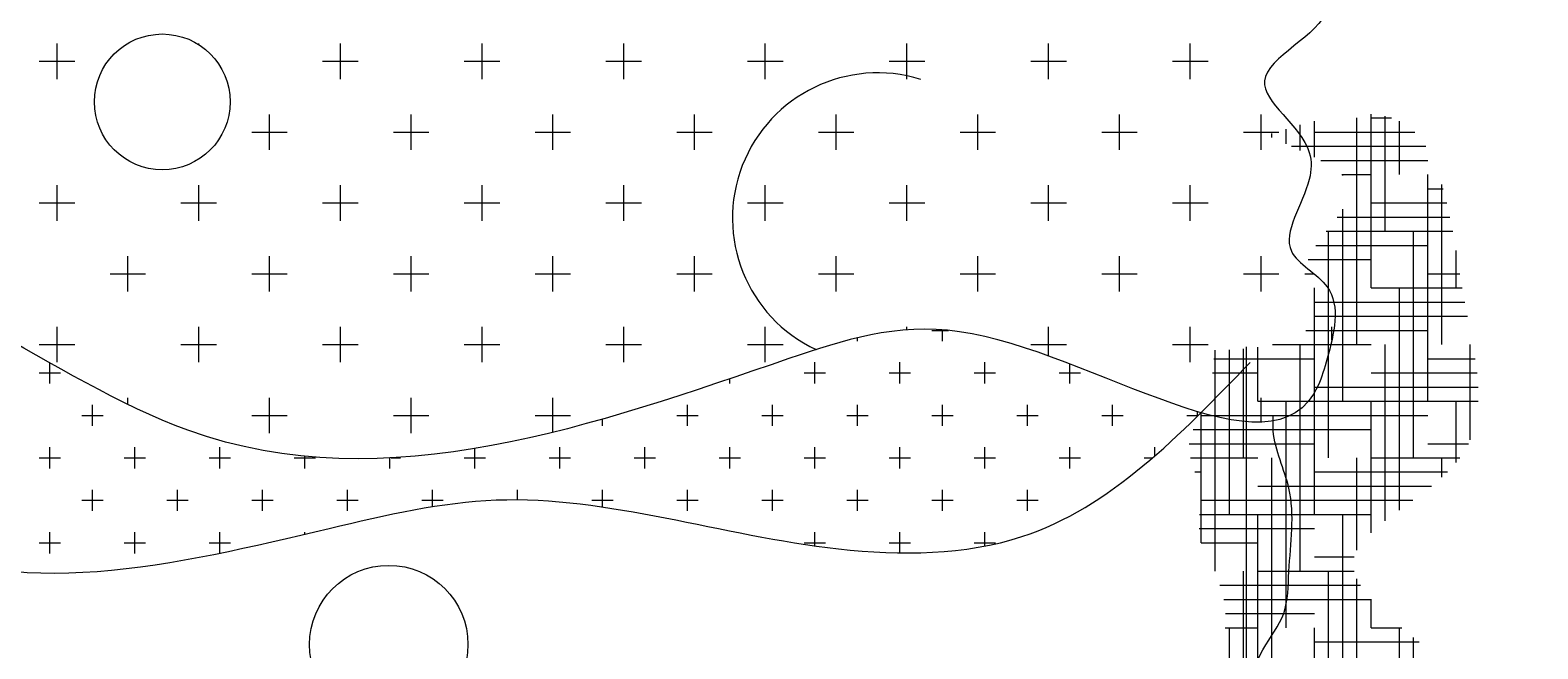
# Model space of a CAD drawing. Units: inches. Extents: x 3731 to 4318, y 1310 to 2388.
# Tile 53 of 57: x 4157 to 4212, y 2274 to 2296. Entities that reach past the tile are written whole.
import ezdxf

# ---------------------------------------------------------------- set-up
doc = ezdxf.new("R2010")
doc.units = ezdxf.units.IN
doc.layers.add('A-ANNO-DIMS', color=2, linetype='Continuous', lineweight=18)
doc.layers.add('A-FURN', color=8, linetype='Continuous', lineweight=13)
doc.styles.get("Standard").update_dxf_attribs({"font": 'arial.ttf'})
doc.dimstyles.get("Standard").update_dxf_attribs({"dimtxt": 0.18, "dimasz": 0.18, "dimexe": 0.18, "dimexo": 0.0625, "dimgap": 0.09, "dimtad": 0, "dimtih": 1, "dimtoh": 1, "dimdec": 4, "dimzin": 0, "dimdsep": 46, "dimtxsty": 'Standard', "dimcen": 0.09, "dimadec": 0, "dimazin": 0, "dimtfac": 1, "dimtdec": 4, "dimtofl": 0, "dimtmove": 0, "dimatfit": 3, "dimfxl": 1, "dimtolj": 1, "dimtzin": 0, "dimarcsym": 0})

# ---------------------------------------------------------------- blocks, each defined once
blk = doc.blocks.new('A$C200C7901')
at = {"linetype": 'ByBlock'}
for p, q in [((0.9504, 1.532), (0.9504, 1.5633)), ((0.9504, 1.532), (0.9504, 1.5633)), ((1.2004, 1.532), (1.2004, 1.5633)), ((1.2004, 1.532), (1.2004, 1.5633)), ((1.3254, 1.532), (1.3254, 1.5633)), ((1.3254, 1.532), (1.3254, 1.5633)), ((1.4504, 1.532), (1.4504, 1.5633)), ((1.4504, 1.532), (1.4504, 1.5633)), ((1.5754, 1.532), (1.5754, 1.5633)), ((1.5754, 1.532), (1.5754, 1.5633)), ((1.7004, 1.532), (1.7004, 1.5633)), ((1.7004, 1.532), (1.7004, 1.5633)), ((1.8254, 1.532), (1.8254, 1.5633)), ((1.8254, 1.532), (1.8254, 1.5633)), ((1.9504, 1.532), (1.9504, 1.5633)), ((1.9504, 1.532), (1.9504, 1.5633)), ((0.9347, 1.5477), (0.966, 1.5477)), ((0.9347, 1.5477), (0.966, 1.5477)), ((1.1847, 1.5477), (1.216, 1.5477)), ((1.1847, 1.5477), (1.216, 1.5477)), ((1.3097, 1.5477), (1.341, 1.5477)), ((1.3097, 1.5477), (1.341, 1.5477)), ((1.4347, 1.5477), (1.466, 1.5477)), ((1.4347, 1.5477), (1.466, 1.5477)), ((1.5597, 1.5477), (1.591, 1.5477)), ((1.5597, 1.5477), (1.591, 1.5477)), ((1.6847, 1.5477), (1.716, 1.5477)), ((1.6847, 1.5477), (1.716, 1.5477)), ((1.8097, 1.5477), (1.841, 1.5477)), ((1.8097, 1.5477), (1.841, 1.5477)), ((1.9347, 1.5477), (1.966, 1.5477)), ((1.9347, 1.5477), (1.966, 1.5477)), ((1.1379, 1.4695), (1.1379, 1.5008)), ((1.1379, 1.4695), (1.1379, 1.5008)), ((1.2629, 1.4695), (1.2629, 1.5008)), ((1.2629, 1.4695), (1.2629, 1.5008)), ((1.3879, 1.4695), (1.3879, 1.5008)), ((1.3879, 1.4695), (1.3879, 1.5008)), ((1.5129, 1.4695), (1.5129, 1.5008)), ((1.5129, 1.4695), (1.5129, 1.5008)), ((1.6379, 1.4695), (1.6379, 1.5008)), ((1.6379, 1.4695), (1.6379, 1.5008)), ((1.7629, 1.4695), (1.7629, 1.5008)), ((1.7629, 1.4695), (1.7629, 1.5008)), ((1.8879, 1.4695), (1.8879, 1.5008)), ((1.8879, 1.4695), (1.8879, 1.5008)), ((2.0129, 1.4695), (2.0129, 1.5008)), ((2.0129, 1.4695), (2.0129, 1.5008)), ((2.0474, 1.4691), (2.0474, 1.4915)), ((2.0474, 1.4691), (2.0474, 1.4915)), ((2.0599, 1.4631), (2.0599, 1.4948)), ((2.0599, 1.4631), (2.0599, 1.4948)), ((2.0974, 1.2977), (2.0974, 1.4977)), ((2.0974, 1.2977), (2.0974, 1.4977)), ((2.1099, 1.3477), (2.1099, 1.5009)), ((2.1099, 1.3477), (2.1099, 1.5009)), ((2.1099, 1.4977), (2.1279, 1.4977)), ((2.1099, 1.4977), (2.1279, 1.4977)), ((2.1224, 1.3977), (2.1224, 1.4992)), ((2.1224, 1.3977), (2.1224, 1.4992)), ((2.1349, 1.4477), (2.1349, 1.4949)), ((2.1349, 1.4477), (2.1349, 1.4949)), ((1.1222, 1.4852), (1.1535, 1.4852)), ((1.1222, 1.4852), (1.1535, 1.4852)), ((1.2472, 1.4852), (1.2785, 1.4852)), ((1.2472, 1.4852), (1.2785, 1.4852)), ((1.3722, 1.4852), (1.4035, 1.4852)), ((1.3722, 1.4852), (1.4035, 1.4852)), ((1.4972, 1.4852), (1.5285, 1.4852)), ((1.4972, 1.4852), (1.5285, 1.4852)), ((1.6222, 1.4852), (1.6535, 1.4852)), ((1.6222, 1.4852), (1.6535, 1.4852)), ((1.7472, 1.4852), (1.7785, 1.4852)), ((1.7472, 1.4852), (1.7785, 1.4852)), ((1.8722, 1.4852), (1.9035, 1.4852)), ((1.8722, 1.4852), (1.9035, 1.4852)), ((1.9972, 1.4852), (2.0285, 1.4852)), ((1.9972, 1.4852), (2.0285, 1.4852)), ((2.0224, 1.4805), (2.0224, 1.4839)), ((2.0224, 1.4805), (2.0224, 1.4839)), ((2.0349, 1.4748), (2.0349, 1.4879)), ((2.0349, 1.4748), (2.0349, 1.4879)), ((2.0599, 1.4852), (2.1484, 1.4852)), ((2.0599, 1.4852), (2.1484, 1.4852)), ((2.0397, 1.4727), (2.1581, 1.4727)), ((2.0397, 1.4727), (2.1581, 1.4727)), ((2.0656, 1.4602), (2.1599, 1.4602)), ((2.0656, 1.4602), (2.1599, 1.4602)), ((0.9504, 1.407), (0.9504, 1.4383)), ((0.9504, 1.407), (0.9504, 1.4383)), ((1.0754, 1.407), (1.0754, 1.4383)), ((1.0754, 1.407), (1.0754, 1.4383)), ((1.2004, 1.407), (1.2004, 1.4383)), ((1.2004, 1.407), (1.2004, 1.4383)), ((1.3254, 1.407), (1.3254, 1.4383)), ((1.3254, 1.407), (1.3254, 1.4383)), ((1.4504, 1.407), (1.4504, 1.4383)), ((1.4504, 1.407), (1.4504, 1.4383)), ((1.5754, 1.407), (1.5754, 1.4383)), ((1.5754, 1.407), (1.5754, 1.4383)), ((1.7004, 1.407), (1.7004, 1.4383)), ((1.7004, 1.407), (1.7004, 1.4383)), ((1.8254, 1.407), (1.8254, 1.4383)), ((1.8254, 1.407), (1.8254, 1.4383)), ((1.9504, 1.407), (1.9504, 1.4383)), ((1.9504, 1.407), (1.9504, 1.4383)), ((2.084, 1.4477), (2.1099, 1.4477)), ((2.084, 1.4477), (2.1099, 1.4477)), ((2.0849, 1.4468), (2.0849, 1.4477)), ((2.0849, 1.4468), (2.0849, 1.4477)), ((2.1599, 1.2477), (2.1599, 1.4477)), ((2.1599, 1.2477), (2.1599, 1.4477)), ((2.1724, 1.2977), (2.1724, 1.439)), ((2.1724, 1.2977), (2.1724, 1.439)), ((2.1599, 1.4352), (2.1735, 1.4352)), ((2.1599, 1.4352), (2.1735, 1.4352)), ((0.9347, 1.4227), (0.966, 1.4227)), ((0.9347, 1.4227), (0.966, 1.4227)), ((1.0597, 1.4227), (1.091, 1.4227)), ((1.0597, 1.4227), (1.091, 1.4227)), ((1.1847, 1.4227), (1.216, 1.4227)), ((1.1847, 1.4227), (1.216, 1.4227)), ((1.3097, 1.4227), (1.341, 1.4227)), ((1.3097, 1.4227), (1.341, 1.4227)), ((1.4347, 1.4227), (1.466, 1.4227)), ((1.4347, 1.4227), (1.466, 1.4227)), ((1.5597, 1.4227), (1.591, 1.4227)), ((1.5597, 1.4227), (1.591, 1.4227)), ((1.6847, 1.4227), (1.716, 1.4227)), ((1.6847, 1.4227), (1.716, 1.4227)), ((1.8097, 1.4227), (1.841, 1.4227)), ((1.8097, 1.4227), (1.841, 1.4227)), ((1.9347, 1.4227), (1.966, 1.4227)), ((1.9347, 1.4227), (1.966, 1.4227)), ((2.08, 1.4102), (2.1795, 1.4102)), ((2.08, 1.4102), (2.1795, 1.4102)), ((2.0849, 1.2477), (2.0849, 1.4171)), ((2.0849, 1.2477), (2.0849, 1.4171)), ((2.1099, 1.4227), (2.1767, 1.4227)), ((2.1099, 1.4227), (2.1767, 1.4227)), ((2.0703, 1.3977), (2.1819, 1.3977)), ((2.0703, 1.3977), (2.1819, 1.3977)), ((2.0724, 1.1977), (2.0724, 1.3977)), ((2.0724, 1.1977), (2.0724, 1.3977)), ((2.1474, 1.1977), (2.1474, 1.3977)), ((2.1474, 1.1977), (2.1474, 1.3977)), ((2.0612, 1.3852), (2.1599, 1.3852)), ((2.0612, 1.3852), (2.1599, 1.3852)), ((1.0129, 1.3445), (1.0129, 1.3758)), ((1.0129, 1.3445), (1.0129, 1.3758)), ((1.1379, 1.3445), (1.1379, 1.3758)), ((1.1379, 1.3445), (1.1379, 1.3758)), ((1.2629, 1.3445), (1.2629, 1.3758)), ((1.2629, 1.3445), (1.2629, 1.3758)), ((1.3879, 1.3445), (1.3879, 1.3758)), ((1.3879, 1.3445), (1.3879, 1.3758)), ((1.5129, 1.3445), (1.5129, 1.3758)), ((1.5129, 1.3445), (1.5129, 1.3758)), ((1.6379, 1.3445), (1.6379, 1.3758)), ((1.6379, 1.3445), (1.6379, 1.3758)), ((1.7629, 1.3445), (1.7629, 1.3758)), ((1.7629, 1.3445), (1.7629, 1.3758)), ((1.8879, 1.3445), (1.8879, 1.3758)), ((1.8879, 1.3445), (1.8879, 1.3758)), ((2.0129, 1.3445), (2.0129, 1.3758)), ((2.0129, 1.3445), (2.0129, 1.3758)), ((2.0545, 1.3727), (2.1099, 1.3727)), ((2.0545, 1.3727), (2.1099, 1.3727)), ((2.1849, 1.3477), (2.1849, 1.3808)), ((2.1849, 1.3477), (2.1849, 1.3808)), ((0.9972, 1.3602), (1.0285, 1.3602)), ((0.9972, 1.3602), (1.0285, 1.3602)), ((1.1222, 1.3602), (1.1535, 1.3602)), ((1.1222, 1.3602), (1.1535, 1.3602)), ((1.2472, 1.3602), (1.2785, 1.3602)), ((1.2472, 1.3602), (1.2785, 1.3602)), ((1.3722, 1.3602), (1.4035, 1.3602)), ((1.3722, 1.3602), (1.4035, 1.3602)), ((1.4972, 1.3602), (1.5285, 1.3602)), ((1.4972, 1.3602), (1.5285, 1.3602)), ((1.6222, 1.3602), (1.6535, 1.3602)), ((1.6222, 1.3602), (1.6535, 1.3602)), ((1.7472, 1.3602), (1.7785, 1.3602)), ((1.7472, 1.3602), (1.7785, 1.3602)), ((1.8722, 1.3602), (1.9035, 1.3602)), ((1.8722, 1.3602), (1.9035, 1.3602)), ((1.9972, 1.3602), (2.0285, 1.3602)), ((1.9972, 1.3602), (2.0285, 1.3602)), ((2.0515, 1.3602), (2.0599, 1.3602)), ((2.0515, 1.3602), (2.0599, 1.3602)), ((2.1599, 1.3602), (2.1883, 1.3602)), ((2.1599, 1.3602), (2.1883, 1.3602)), ((2.0599, 1.1477), (2.0599, 1.3477)), ((2.0599, 1.1477), (2.0599, 1.3477)), ((2.1099, 1.3477), (2.1904, 1.3477)), ((2.1099, 1.3477), (2.1904, 1.3477)), ((2.1349, 1.1515), (2.1349, 1.3477)), ((2.1349, 1.1515), (2.1349, 1.3477)), ((2.0599, 1.3352), (2.1926, 1.3352)), ((2.0599, 1.3352), (2.1926, 1.3352)), ((2.0594, 1.3227), (2.195, 1.3227)), ((2.0594, 1.3227), (2.195, 1.3227)), ((0.9504, 1.282), (0.9504, 1.3133)), ((0.9504, 1.282), (0.9504, 1.3133)), ((1.0754, 1.282), (1.0754, 1.3133)), ((1.0754, 1.282), (1.0754, 1.3133)), ((1.2004, 1.282), (1.2004, 1.3133)), ((1.2004, 1.282), (1.2004, 1.3133)), ((1.3254, 1.282), (1.3254, 1.3133)), ((1.3254, 1.282), (1.3254, 1.3133)), ((1.4504, 1.282), (1.4504, 1.3133)), ((1.4504, 1.282), (1.4504, 1.3133)), ((1.5754, 1.282), (1.5754, 1.3133)), ((1.5754, 1.282), (1.5754, 1.3133)), ((1.7004, 1.3106), (1.7004, 1.3133)), ((1.7004, 1.3106), (1.7004, 1.3133)), ((1.7222, 1.3102), (1.7369, 1.3102)), ((1.7222, 1.3102), (1.7369, 1.3102)), ((1.7316, 1.3008), (1.7316, 1.3106)), ((1.7316, 1.3008), (1.7316, 1.3106)), ((1.8254, 1.2876), (1.8254, 1.3133)), ((1.8254, 1.2876), (1.8254, 1.3133)), ((1.9504, 1.282), (1.9504, 1.3133)), ((1.9504, 1.282), (1.9504, 1.3133)), ((2.0524, 1.3102), (2.1599, 1.3102)), ((2.0524, 1.3102), (2.1599, 1.3102)), ((2.0754, 1.3017), (2.0754, 1.3133)), ((2.0754, 1.3017), (2.0754, 1.3133)), ((0.9347, 1.2977), (0.966, 1.2977)), ((0.9347, 1.2977), (0.966, 1.2977)), ((1.0597, 1.2977), (1.091, 1.2977)), ((1.0597, 1.2977), (1.091, 1.2977)), ((1.1847, 1.2977), (1.216, 1.2977)), ((1.1847, 1.2977), (1.216, 1.2977)), ((1.3097, 1.2977), (1.341, 1.2977)), ((1.3097, 1.2977), (1.341, 1.2977)), ((1.4347, 1.2977), (1.466, 1.2977)), ((1.4347, 1.2977), (1.466, 1.2977)), ((1.5597, 1.2977), (1.591, 1.2977)), ((1.5597, 1.2977), (1.591, 1.2977)), ((1.6566, 1.3008), (1.6566, 1.3036)), ((1.6566, 1.3008), (1.6566, 1.3036)), ((1.8097, 1.2977), (1.841, 1.2977)), ((1.8097, 1.2977), (1.841, 1.2977)), ((1.9347, 1.2977), (1.966, 1.2977)), ((1.9347, 1.2977), (1.966, 1.2977)), ((1.9724, 1.0977), (1.9724, 1.2927)), ((1.9724, 1.0977), (1.9724, 1.2927)), ((1.9849, 1.1477), (1.9849, 1.293)), ((1.9849, 1.1477), (1.9849, 1.293)), ((1.9974, 1.1977), (1.9974, 1.2939)), ((1.9974, 1.1977), (1.9974, 1.2939)), ((2.0099, 1.2477), (2.0099, 1.2953)), ((2.0099, 1.2477), (2.0099, 1.2953)), ((2.023, 1.2977), (2.1099, 1.2977)), ((2.023, 1.2977), (2.1099, 1.2977)), ((2.0474, 1.0977), (2.0474, 1.2977)), ((2.0474, 1.0977), (2.0474, 1.2977)), ((2.0597, 1.2977), (2.0744, 1.2977)), ((2.0597, 1.2977), (2.0744, 1.2977)), ((2.1224, 1.1421), (2.1224, 1.2977)), ((2.1224, 1.1421), (2.1224, 1.2977)), ((2.1974, 1.2135), (2.1974, 1.2977)), ((2.1974, 1.2135), (2.1974, 1.2977)), ((0.9441, 1.2633), (0.9441, 1.2816)), ((0.9441, 1.2633), (0.9441, 1.2816)), ((1.6191, 1.2633), (1.6191, 1.282)), ((1.6191, 1.2633), (1.6191, 1.282)), ((1.6941, 1.2633), (1.6941, 1.282)), ((1.6941, 1.2633), (1.6941, 1.282)), ((1.7691, 1.2633), (1.7691, 1.282)), ((1.7691, 1.2633), (1.7691, 1.282)), ((1.8441, 1.2633), (1.8441, 1.2806)), ((1.8441, 1.2633), (1.8441, 1.2806)), ((1.9711, 1.2852), (2.0599, 1.2852)), ((1.9711, 1.2852), (2.0599, 1.2852)), ((2.1599, 1.2852), (2.2018, 1.2852)), ((2.1599, 1.2852), (2.2018, 1.2852)), ((0.9347, 1.2727), (0.9535, 1.2727)), ((0.9347, 1.2727), (0.9535, 1.2727)), ((1.5441, 1.2633), (1.5441, 1.2675)), ((1.5441, 1.2633), (1.5441, 1.2675)), ((1.6097, 1.2727), (1.6285, 1.2727)), ((1.6097, 1.2727), (1.6285, 1.2727)), ((1.6847, 1.2727), (1.7035, 1.2727)), ((1.6847, 1.2727), (1.7035, 1.2727)), ((1.7597, 1.2727), (1.7785, 1.2727)), ((1.7597, 1.2727), (1.7785, 1.2727)), ((1.8347, 1.2727), (1.8535, 1.2727)), ((1.8347, 1.2727), (1.8535, 1.2727)), ((1.97, 1.2727), (2.0099, 1.2727)), ((1.97, 1.2727), (2.0099, 1.2727)), ((2.1099, 1.2727), (2.2034, 1.2727)), ((2.1099, 1.2727), (2.2034, 1.2727)), ((1.0129, 1.2448), (1.0129, 1.2508)), ((1.0129, 1.2448), (1.0129, 1.2508)), ((1.1379, 1.2195), (1.1379, 1.2508)), ((1.1379, 1.2195), (1.1379, 1.2508)), ((1.2629, 1.2195), (1.2629, 1.2508)), ((1.2629, 1.2195), (1.2629, 1.2508)), ((1.3879, 1.2202), (1.3879, 1.2508)), ((1.3879, 1.2202), (1.3879, 1.2508)), ((2.0129, 1.2293), (2.0129, 1.2508)), ((2.0129, 1.2293), (2.0129, 1.2508)), ((2.0599, 1.2602), (2.2044, 1.2602)), ((2.0599, 1.2602), (2.2044, 1.2602)), ((0.9816, 1.2258), (0.9816, 1.2445)), ((0.9816, 1.2258), (0.9816, 1.2445)), ((1.5066, 1.2258), (1.5066, 1.2445)), ((1.5066, 1.2258), (1.5066, 1.2445)), ((1.5816, 1.2258), (1.5816, 1.2445)), ((1.5816, 1.2258), (1.5816, 1.2445)), ((1.6566, 1.2258), (1.6566, 1.2445)), ((1.6566, 1.2258), (1.6566, 1.2445)), ((1.7316, 1.2258), (1.7316, 1.2445)), ((1.7316, 1.2258), (1.7316, 1.2445)), ((1.8066, 1.2258), (1.8066, 1.2445)), ((1.8066, 1.2258), (1.8066, 1.2445)), ((1.8816, 1.2258), (1.8816, 1.2445)), ((1.8816, 1.2258), (1.8816, 1.2445)), ((1.9566, 1.2344), (1.9566, 1.2385)), ((1.9566, 1.2344), (1.9566, 1.2385)), ((1.9599, 1.1228), (1.9599, 1.2373)), ((1.9599, 1.1228), (1.9599, 1.2373)), ((2.0099, 1.2477), (2.2045, 1.2477)), ((2.0099, 1.2477), (2.2045, 1.2477)), ((2.0349, 1.0477), (2.0349, 1.2477)), ((2.0349, 1.0477), (2.0349, 1.2477)), ((2.1099, 1.1315), (2.1099, 1.2477)), ((2.1099, 1.1315), (2.1099, 1.2477)), ((2.1849, 1.1935), (2.1849, 1.2477)), ((2.1849, 1.1935), (2.1849, 1.2477)), ((0.9722, 1.2352), (0.991, 1.2352)), ((0.9722, 1.2352), (0.991, 1.2352)), ((1.1222, 1.2352), (1.1535, 1.2352)), ((1.1222, 1.2352), (1.1535, 1.2352)), ((1.2472, 1.2352), (1.2785, 1.2352)), ((1.2472, 1.2352), (1.2785, 1.2352)), ((1.3722, 1.2352), (1.4035, 1.2352)), ((1.3722, 1.2352), (1.4035, 1.2352)), ((1.4316, 1.2258), (1.4316, 1.2318)), ((1.4316, 1.2258), (1.4316, 1.2318)), ((1.4972, 1.2352), (1.516, 1.2352)), ((1.4972, 1.2352), (1.516, 1.2352)), ((1.5722, 1.2352), (1.591, 1.2352)), ((1.5722, 1.2352), (1.591, 1.2352)), ((1.6472, 1.2352), (1.666, 1.2352)), ((1.6472, 1.2352), (1.666, 1.2352)), ((1.7222, 1.2352), (1.741, 1.2352)), ((1.7222, 1.2352), (1.741, 1.2352)), ((1.7972, 1.2352), (1.816, 1.2352)), ((1.7972, 1.2352), (1.816, 1.2352)), ((1.8722, 1.2352), (1.891, 1.2352)), ((1.8722, 1.2352), (1.891, 1.2352)), ((1.9472, 1.2352), (1.9574, 1.2352)), ((1.9472, 1.2352), (1.9574, 1.2352)), ((1.9599, 1.2352), (2.1599, 1.2352)), ((1.9599, 1.2352), (2.1599, 1.2352)), ((2, 1.2352), (2.0285, 1.2352)), ((2, 1.2352), (2.0285, 1.2352)), ((1.953, 1.2227), (2.1099, 1.2227)), ((1.953, 1.2227), (2.1099, 1.2227)), ((0.9347, 1.1977), (0.9535, 1.1977)), ((0.9347, 1.1977), (0.9535, 1.1977)), ((0.9441, 1.1883), (0.9441, 1.207)), ((0.9441, 1.1883), (0.9441, 1.207)), ((1.0097, 1.1977), (1.0285, 1.1977)), ((1.0097, 1.1977), (1.0285, 1.1977)), ((1.0191, 1.1883), (1.0191, 1.207)), ((1.0191, 1.1883), (1.0191, 1.207)), ((1.0847, 1.1977), (1.1035, 1.1977)), ((1.0847, 1.1977), (1.1035, 1.1977)), ((1.0941, 1.1883), (1.0941, 1.207)), ((1.0941, 1.1883), (1.0941, 1.207)), ((1.1597, 1.1977), (1.1785, 1.1977)), ((1.1597, 1.1977), (1.1785, 1.1977)), ((1.1691, 1.1883), (1.1691, 1.1991)), ((1.1691, 1.1883), (1.1691, 1.1991)), ((1.2441, 1.1883), (1.2441, 1.1976)), ((1.2441, 1.1883), (1.2441, 1.1976)), ((1.2452, 1.1977), (1.2535, 1.1977)), ((1.2452, 1.1977), (1.2535, 1.1977)), ((1.3097, 1.1977), (1.3285, 1.1977)), ((1.3097, 1.1977), (1.3285, 1.1977)), ((1.3191, 1.1883), (1.3191, 1.2059)), ((1.3191, 1.1883), (1.3191, 1.2059)), ((1.3847, 1.1977), (1.4035, 1.1977)), ((1.3847, 1.1977), (1.4035, 1.1977)), ((1.3941, 1.1883), (1.3941, 1.207)), ((1.3941, 1.1883), (1.3941, 1.207)), ((1.4597, 1.1977), (1.4785, 1.1977)), ((1.4597, 1.1977), (1.4785, 1.1977)), ((1.4691, 1.1883), (1.4691, 1.207)), ((1.4691, 1.1883), (1.4691, 1.207)), ((1.5347, 1.1977), (1.5535, 1.1977)), ((1.5347, 1.1977), (1.5535, 1.1977)), ((1.5441, 1.1883), (1.5441, 1.207)), ((1.5441, 1.1883), (1.5441, 1.207)), ((1.6097, 1.1977), (1.6285, 1.1977)), ((1.6097, 1.1977), (1.6285, 1.1977)), ((1.6191, 1.1883), (1.6191, 1.207)), ((1.6191, 1.1883), (1.6191, 1.207)), ((1.6847, 1.1977), (1.7035, 1.1977)), ((1.6847, 1.1977), (1.7035, 1.1977)), ((1.6941, 1.1883), (1.6941, 1.207)), ((1.6941, 1.1883), (1.6941, 1.207)), ((1.7597, 1.1977), (1.7785, 1.1977)), ((1.7597, 1.1977), (1.7785, 1.1977)), ((1.7691, 1.1883), (1.7691, 1.207)), ((1.7691, 1.1883), (1.7691, 1.207)), ((1.8347, 1.1977), (1.8535, 1.1977)), ((1.8347, 1.1977), (1.8535, 1.1977)), ((1.8441, 1.1883), (1.8441, 1.207)), ((1.8441, 1.1883), (1.8441, 1.207)), ((1.9097, 1.1977), (1.917, 1.1977)), ((1.9097, 1.1977), (1.917, 1.1977)), ((1.9191, 1.1995), (1.9191, 1.207)), ((1.9191, 1.1995), (1.9191, 1.207)), ((1.9495, 1.2102), (2.0599, 1.2102)), ((1.9495, 1.2102), (2.0599, 1.2102)), ((1.9506, 1.1977), (2.0099, 1.1977)), ((1.9506, 1.1977), (2.0099, 1.1977)), ((2.0974, 1.1161), (2.0974, 1.1977)), ((2.0974, 1.1161), (2.0974, 1.1977)), ((2.1099, 1.1977), (2.1882, 1.1977)), ((2.1099, 1.1977), (2.1882, 1.1977)), ((2.1599, 1.2102), (2.1959, 1.2102)), ((2.1599, 1.2102), (2.1959, 1.2102)), ((2.1724, 1.1807), (2.1724, 1.1977)), ((2.1724, 1.1807), (2.1724, 1.1977)), ((1.9545, 1.1852), (1.9599, 1.1852)), ((1.9545, 1.1852), (1.9599, 1.1852)), ((2.0599, 1.1852), (2.1772, 1.1852)), ((2.0599, 1.1852), (2.1772, 1.1852)), ((2.0099, 1.1727), (2.1631, 1.1727)), ((2.0099, 1.1727), (2.1631, 1.1727)), ((0.9722, 1.1602), (0.991, 1.1602)), ((0.9722, 1.1602), (0.991, 1.1602)), ((0.9816, 1.1508), (0.9816, 1.1695)), ((0.9816, 1.1508), (0.9816, 1.1695)), ((1.0472, 1.1602), (1.066, 1.1602)), ((1.0472, 1.1602), (1.066, 1.1602)), ((1.0566, 1.1508), (1.0566, 1.1695)), ((1.0566, 1.1508), (1.0566, 1.1695)), ((1.1222, 1.1602), (1.141, 1.1602)), ((1.1222, 1.1602), (1.141, 1.1602)), ((1.1316, 1.1508), (1.1316, 1.1695)), ((1.1316, 1.1508), (1.1316, 1.1695)), ((1.1972, 1.1602), (1.216, 1.1602)), ((1.1972, 1.1602), (1.216, 1.1602)), ((1.2066, 1.1508), (1.2066, 1.1695)), ((1.2066, 1.1508), (1.2066, 1.1695)), ((1.2722, 1.1602), (1.291, 1.1602)), ((1.2722, 1.1602), (1.291, 1.1602)), ((1.2816, 1.1547), (1.2816, 1.1695)), ((1.2816, 1.1547), (1.2816, 1.1695)), ((1.3566, 1.1608), (1.3566, 1.1695)), ((1.3566, 1.1608), (1.3566, 1.1695)), ((1.4222, 1.1602), (1.441, 1.1602)), ((1.4222, 1.1602), (1.441, 1.1602)), ((1.4316, 1.1544), (1.4316, 1.1695)), ((1.4316, 1.1544), (1.4316, 1.1695)), ((1.4972, 1.1602), (1.516, 1.1602)), ((1.4972, 1.1602), (1.516, 1.1602)), ((1.5066, 1.1508), (1.5066, 1.1695)), ((1.5066, 1.1508), (1.5066, 1.1695)), ((1.5722, 1.1602), (1.591, 1.1602)), ((1.5722, 1.1602), (1.591, 1.1602)), ((1.5816, 1.1508), (1.5816, 1.1695)), ((1.5816, 1.1508), (1.5816, 1.1695)), ((1.6472, 1.1602), (1.666, 1.1602)), ((1.6472, 1.1602), (1.666, 1.1602)), ((1.6566, 1.1508), (1.6566, 1.1695)), ((1.6566, 1.1508), (1.6566, 1.1695)), ((1.7222, 1.1602), (1.741, 1.1602)), ((1.7222, 1.1602), (1.741, 1.1602)), ((1.7316, 1.1508), (1.7316, 1.1695)), ((1.7316, 1.1508), (1.7316, 1.1695)), ((1.7972, 1.1602), (1.816, 1.1602)), ((1.7972, 1.1602), (1.816, 1.1602)), ((1.8066, 1.1508), (1.8066, 1.1695)), ((1.8066, 1.1508), (1.8066, 1.1695)), ((1.9599, 1.1602), (2.1468, 1.1602)), ((1.9599, 1.1602), (2.1468, 1.1602)), ((1.9585, 1.1477), (2.1099, 1.1477)), ((1.9585, 1.1477), (2.1099, 1.1477)), ((2.0099, 0.9477), (2.0099, 1.1477)), ((2.0099, 0.9477), (2.0099, 1.1477)), ((2.0849, 0.9477), (2.0849, 1.1477)), ((2.0849, 0.9477), (2.0849, 1.1477)), ((0.9441, 1.1133), (0.9441, 1.132)), ((0.9441, 1.1133), (0.9441, 1.132)), ((1.0191, 1.1133), (1.0191, 1.132)), ((1.0191, 1.1133), (1.0191, 1.132)), ((1.0941, 1.1136), (1.0941, 1.132)), ((1.0941, 1.1136), (1.0941, 1.132)), ((1.1691, 1.1303), (1.1691, 1.132)), ((1.1691, 1.1303), (1.1691, 1.132)), ((1.6191, 1.1201), (1.6191, 1.132)), ((1.6191, 1.1201), (1.6191, 1.132)), ((1.6941, 1.1139), (1.6941, 1.132)), ((1.6941, 1.1139), (1.6941, 1.132)), ((1.7691, 1.1198), (1.7691, 1.132)), ((1.7691, 1.1198), (1.7691, 1.132)), ((1.9581, 1.1352), (2.0599, 1.1352)), ((1.9581, 1.1352), (2.0599, 1.1352)), ((0.9347, 1.1227), (0.9535, 1.1227)), ((0.9347, 1.1227), (0.9535, 1.1227)), ((1.0097, 1.1227), (1.0285, 1.1227)), ((1.0097, 1.1227), (1.0285, 1.1227)), ((1.0847, 1.1227), (1.1035, 1.1227)), ((1.0847, 1.1227), (1.1035, 1.1227)), ((1.6097, 1.1227), (1.6285, 1.1227)), ((1.6097, 1.1227), (1.6285, 1.1227)), ((1.6847, 1.1227), (1.7035, 1.1227)), ((1.6847, 1.1227), (1.7035, 1.1227)), ((1.7597, 1.1227), (1.7785, 1.1227)), ((1.7597, 1.1227), (1.7785, 1.1227)), ((1.9599, 1.1227), (2.0099, 1.1227)), ((1.9599, 1.1227), (2.0099, 1.1227)), ((2.0599, 1.1102), (2.0951, 1.1102)), ((2.0599, 1.1102), (2.0951, 1.1102)), ((1.9974, 0.8977), (1.9974, 1.0977)), ((1.9974, 0.8977), (1.9974, 1.0977)), ((2.0099, 1.0977), (2.095, 1.0977)), ((2.0099, 1.0977), (2.095, 1.0977)), ((2.0724, 0.8977), (2.0724, 1.0977)), ((2.0724, 0.8977), (2.0724, 1.0977)), ((2.0974, 0.9977), (2.0974, 1.0909)), ((2.0974, 0.9977), (2.0974, 1.0909)), ((1.9763, 1.0852), (2.1005, 1.0852)), ((1.9763, 1.0852), (2.1005, 1.0852)), ((1.9799, 1.0727), (2.1099, 1.0727)), ((1.9799, 1.0727), (2.1099, 1.0727)), ((2.1099, 1.0477), (2.1099, 1.0729)), ((2.1099, 1.0477), (2.1099, 1.0729)), ((1.9815, 1.0602), (2.0599, 1.0602)), ((1.9815, 1.0602), (2.0599, 1.0602)), ((1.981, 1.0477), (2.0099, 1.0477)), ((1.981, 1.0477), (2.0099, 1.0477)), ((1.9849, 0.9171), (1.9849, 1.0477)), ((1.9849, 0.9171), (1.9849, 1.0477)), ((2.0599, 0.8477), (2.0599, 1.0477)), ((2.0599, 0.8477), (2.0599, 1.0477)), ((2.1099, 1.0477), (2.137, 1.0477)), ((2.1099, 1.0477), (2.137, 1.0477)), ((2.1349, 0.8477), (2.1349, 1.0477)), ((2.1349, 0.8477), (2.1349, 1.0477)), ((2.1474, 0.8977), (2.1474, 1.0391)), ((2.1474, 0.8977), (2.1474, 1.0391)), ((2.0599, 1.0352), (2.1523, 1.0352)), ((2.0599, 1.0352), (2.1523, 1.0352))]:
    blk.add_line(p, q, dxfattribs=at)
for p, q in [((1.0754, 1.5625), (1.0754, 1.5633)), ((1.0754, 1.5625), (1.0754, 1.5633)), ((2, 0.2957), (2, 1.2957)), ((2.0224, 0.9977), (2.0224, 1.1977)), ((2.0224, 0.9977), (2.0224, 1.1977))]:
    blk.add_line(p, q)
for centre, radius in [((1.0433, 1.5119), 0.0599), ((1.2431, 1.0329), 0.0699)]:
    blk.add_circle(centre, radius)
blk.add_arc((1.6746, 1.4093), 0.1282, 72.7909, 244.8695, dxfattribs=at)
blk.add_arc((1.6746, 1.4093), 0.1282, 72.7909, 244.8695, dxfattribs=at)
for points, knots in [([(0.4485, 1.7835), (0.4321, 1.7496), (0.4062, 1.6964), (0.49, 1.6713), (0.4719, 1.5969), (0.4123, 1.592), (0.4233, 1.5337), (0.4954, 1.5086), (0.4012, 1.4738), (0.3253, 1.4306), (0.4113, 1.3764), (0.3688, 1.3065), (0.5579, 1.2663), (0.741, 1.4533), (1.1127, 1.1109), (1.4811, 1.2478), (1.7885, 1.3492), (2.0357, 1.1637), (2.0748, 1.2974), (2.0876, 1.349), (2.0192, 1.3805), (2.0564, 1.4298), (2.0588, 1.4846), (1.9759, 1.5349), (2.1004, 1.5845), (2.0397, 1.6519), (1.971, 1.7053), (2.1104, 1.8981), (1.5946, 1.7967), (1.2448, 1.7472), (0.8129, 1.7935), (0.4953, 1.8548), (0.4582, 1.7983), (0.4485, 1.7835)], [0, 0, 0, 0, 88.420092, 139.08588, 204.302936, 239.695496, 287.801042, 327.365471, 412.960499, 463.626286, 552.059846, 584.668336, 662.614915, 940.993281, 1309.926334, 1844.022653, 1996.276242, 2316.43048, 2341.441004, 2404.707416, 2449.463774, 2514.680778, 2538.40571, 2613.031547, 2697.13096, 2760.903931, 2822.692699, 2945.47, 3215.060018, 3725.584917, 4361.974444, 4504.671998, 4555.32777, 4555.32777, 4555.32777, 4555.32777]), ([(0.4856, 1.3429), (0.5504, 1.3182), (0.6715, 1.2721), (0.8374, 1.0498), (1.1164, 1.1183), (1.3878, 1.1816), (1.5888, 1.1102), (1.8403, 1.1127), (1.9415, 1.2178), (2.0032, 1.2819)], [0, 0, 0, 0, 205.411753, 383.654933, 772.067458, 921.644661, 1226.793228, 1388.983508, 1642.292305, 1642.292305, 1642.292305, 1642.292305])]:
    blk.add_open_spline(points, degree=3, knots=knots)
blk.add_open_spline([(0.473, 1.2954), (0.4739, 1.2781), (0.4755, 1.2477), (0.5032, 1.2084), (0.4801, 1.1701), (0.4928, 1.1255), (0.4674, 1.0912), (0.4579, 1.0351), (0.501, 0.9724), (0.4311, 0.8832), (0.4902, 0.8637), (0.4843, 0.8288), (0.4774, 0.7906), (0.4625, 0.7457), (0.459, 0.6999), (0.4816, 0.6664), (0.4748, 0.625), (0.4791, 0.5889), (0.4533, 0.5528), (0.4738, 0.5004), (0.4658, 0.4502), (0.4696, 0.3946), (0.4189, 0.3935), (0.4493, 0.3684), (0.4694, 0.3857), (0.4922, 0.3576), (0.5297, 0.3262), (0.5917, 0.3353), (0.6454, 0.3754), (0.7083, 0.3741), (0.7643, 0.3328), (0.826, 0.346), (0.925, 0.3388), (1.0353, 0.3593), (1.1561, 0.3744), (1.2477, 0.3154), (1.3302, 0.3474), (1.4086, 0.3512), (1.5217, 0.3878), (1.6362, 0.3176), (1.7682, 0.3285), (1.8402, 0.3019), (1.9071, 0.3529), (1.9647, 0.3412), (2.0795, 0.2948), (2.0472, 0.3498), (2.0343, 0.3772), (2.0435, 0.43), (2.0109, 0.5782), (2.0746, 0.4643), (2.0805, 0.584), (2.0084, 0.5979), (2.0343, 0.6846), (2.0344, 0.746), (2.0293, 0.8096), (2.0489, 0.8545), (2.0652, 0.9218), (1.9842, 0.9297), (2.0007, 1.0162), (2.0367, 1.0585), (2.0367, 1.1102), (2.0457, 1.1647), (2.0226, 1.2084), (2.0234, 1.2306), (2.0236, 1.2352)], degree=3, knots=[0, 0, 0, 0, 51.660678, 90.967412, 128.902454, 170.303599, 219.852997, 247.834962, 336.321557, 429.35469, 458.821847, 477.222321, 524.135809, 581.038434, 617.839381, 657.146115, 693.947125, 740.178081, 760.753248, 820.731705, 885.133458, 928.777044, 953.563729, 976.574207, 995.553042, 1018.563482, 1064.584401, 1147.951297, 1174.787598, 1266.851571, 1308.018447, 1377.066427, 1441.511314, 1608.245014, 1714.11869, 1792.771707, 1913.247991, 1954.931389, 2029.864445, 2259.189419, 2305.221512, 2429.507982, 2456.344283, 2543.92595, 2627.925037, 2662.96218, 2687.736879, 2719.937755, 2839.540991, 2875.47895, 2953.681041, 2993.270313, 3066.872333, 3154.395764, 3200.397042, 3248.426375, 3312.828127, 3347.881398, 3444.484026, 3481.577522, 3518.665244, 3592.267265, 3644.719162, 3658.519501, 3658.519501, 3658.519501, 3658.519501], dxfattribs=at)
blk = doc.blocks.new('*D37')
at = {"layer": 'A-ANNO-DIMS', "color": 0, "lineweight": -2, "transparency": 16777216}
for p, q in [((4239.271, 2338.382), (4318.341, 2338.382)), ((4318.161, 2338.202), (4318.161, 2300.563)), ((4318.161, 2262.562), (4318.161, 2300.2)), ((4103.271, 2262.382), (4318.341, 2262.382))]:
    blk.add_line(p, q, dxfattribs=at)
at = {"layer": 'A-ANNO-DIMS', "color": 0, "transparency": 16777216}
for points in [[(4318.131, 2338.202), (4318.191, 2338.202), (4318.161, 2338.382)], [(4318.131, 2262.562), (4318.191, 2262.562), (4318.161, 2262.382)]]:
    blk.add_solid(points, dxfattribs=at)
at = {"layer": 'Defpoints', "color": 0, "transparency": 16777216}
for p in [(4239.209, 2338.382), (4318.161, 2338.382), (4103.209, 2262.382)]:
    blk.add_point(p, dxfattribs=at)
at = {"layer": 'A-ANNO-DIMS', "color": 0, "transparency": 16777216, "insert": (4318.161, 2300.382), "char_height": 0.18, "attachment_point": 5}
blk.add_mtext('\\A1;76', dxfattribs=at)

msp = doc.modelspace()

# ---------------------------------------------------------------- block references
at = {"layer": 'A-FURN', "xscale": 41.1071563136412, "yscale": 41.1071563136412, "zscale": 41.1071563136412}
msp.add_blockref('A$C200C7901', (4119.004, 2231.625), dxfattribs=at)

# ---------------------------------------------------------------- dimensions: what is measured, and where the dimension line sits
at = {"layer": 'A-ANNO-DIMS'}
dim = msp.add_linear_dim(base=(4318.161, 2338.382), p1=(4103.209, 2262.382), p2=(4239.209, 2338.382), angle=90, dimstyle='Standard', override={"dimdec": 0, "dimlfac": 1, "dimrnd": 0, "dimzin": 0, "dimdsep": 46, "dimlunit": 2}, dxfattribs=at)
dim.commit()
dim.dimension.update_dxf_attribs({"geometry": '*D37', "text_midpoint": (4318.161, 2300.382)})

doc.saveas('drawing.dxf')
